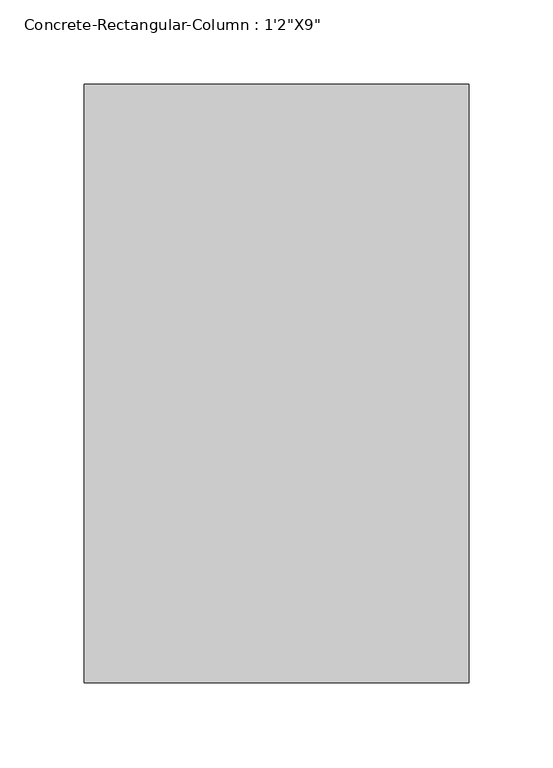
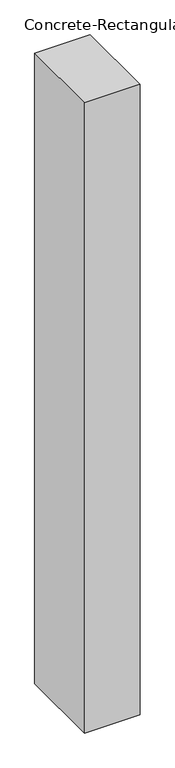
"""IFC4 building model written with IfcOpenShell, lengths in millimetres: column geometry."""

from ifc_helpers import new_model, si_unit, frame, origin, place, context, project, spatial, polyline, outline, extrude, source, transform, mapped, element, save


def column_3693de43(model_context):
    return source(origin(), model_context, "Body", "SweptSolid", [
        extrude(outline(polyline([(114.3, 177.8), (114.3, -177.8), (-114.3, -177.8), (-114.3, 177.8), (114.3, 177.8)])), frame((0.0, 0.0, 16002.0), z_axis=(0.0, 0.0, 1.0), x_axis=(1.0, 0.0, 0.0)), (0.0, 0.0, 1.0), 2743.2),
    ])


if __name__ == "__main__":
    model = new_model("IFC4")
    model_context = context("Model", 3, world=origin())
    ifc_project = project(units=[si_unit("LENGTHUNIT", "METRE", prefix="MILLI")], contexts=[model_context])
    site = spatial("IfcSite", under=ifc_project)
    building = spatial("IfcBuilding", under=site)
    placement = place(None, origin())
    column_shape = column_3693de43(model_context)
    element("IfcColumn", 1, ObjectType="Concrete-Rectangular-Column : 1'2\"X9\"", at=placement, inside=building, context=model_context, shape_type="MappedRepresentation", body=[
        mapped(column_shape, transform((0.0, 0.0, 0.0), x_axis=(1.0, 0.0, 0.0), y_axis=(0.0, 1.0, 0.0), z_axis=(0.0, 0.0, 1.0))),
    ])
    save(model, "model.ifc")

# Revit data of these elements
# Type "Concrete-Rectangular-Column : 1'2\"X9\""
#   Assembly Code = "B10"
#   b = 0' - 9"
#   h = 1' - 2"
#   Structural Material [instance default] = Concrete, Cast-in-Place gray
# Element 1 (IfcColumn, "Concrete-Rectangular-Column : 1'2\"X9\"")
#   Materials on its faces: "Concrete, Cast-in-Place gray"
# Materials
#   "Concrete, Cast-in-Place gray": class "Concrete", colour RGB 192 192 192, transparency 0, Description = "Cast-in-place concrete", Cost = 0
